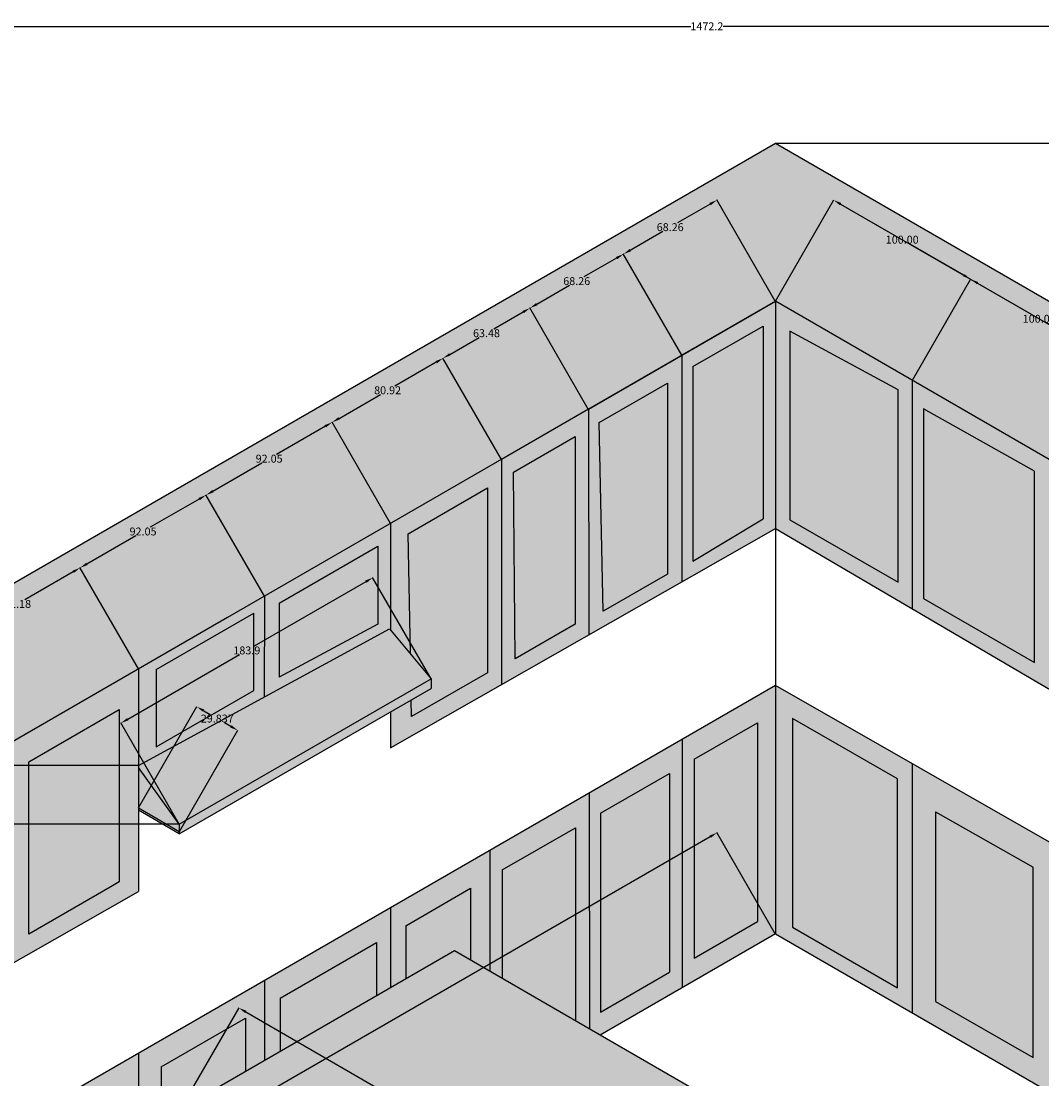
# Model space of a CAD drawing. Units: centimetres. Extents: x -744 to 1642, y 210 to 1375.
# Tile 3 of 8: x -357 to 288, y 707 to 1375. Entities that reach past the tile are written whole.
import ezdxf

# ---------------------------------------------------------------- set-up
doc = ezdxf.new("R2010")
doc.units = ezdxf.units.CM
doc.header["$MEASUREMENT"] = 0
for name, color, linetype, lineweight in [('A-ANNO-DIMS', 2, 'Continuous', 18), ('A-EQPM-PATT', 9, 'Continuous', 13), ('A-FURN', 7, 'Continuous', 25), ('A-FURN-PATT', 30, 'Continuous', 13), ('A-WALL-PATT', 61, 'Continuous', 13)]:
    doc.layers.add(name, color=color, linetype=linetype, lineweight=lineweight)
doc.styles.get("Standard").update_dxf_attribs({"font": 'arial.ttf'})
doc.dimstyles.get("Standard").update_dxf_attribs({"dimtxt": 5, "dimasz": 5, "dimexe": 0.18, "dimexo": 0.0625, "dimgap": 0.09, "dimtad": 0, "dimtih": 1, "dimtoh": 1, "dimdec": 0, "dimzin": 0, "dimdsep": 46, "dimtxsty": 'Standard', "dimcen": 0.09, "dimadec": 0, "dimazin": 0, "dimtfac": 1, "dimtdec": 0, "dimtofl": 0, "dimtmove": 0, "dimatfit": 3, "dimfxl": 1, "dimtolj": 1, "dimtzin": 0, "dimarcsym": 0})

# ---------------------------------------------------------------- blocks, each defined once
blk = doc.blocks.new('*D7')
at = {"layer": 'A-ANNO-DIMS', "color": 0, "lineweight": -2, "transparency": 16777216}
for p, q in [((-659.99, 848.29), (-659.99, 1372.26)), ((-654.99, 1372.08), (65.92, 1372.08)), ((807.25, 1372.08), (86.34, 1372.08)), ((812.25, 898.29), (812.25, 1372.26))]:
    blk.add_line(p, q, dxfattribs=at)
at = {"layer": 'A-ANNO-DIMS', "color": 0, "transparency": 16777216}
for points in [[(-654.99, 1372.91), (-654.99, 1371.25), (-659.99, 1372.08)], [(807.25, 1372.91), (807.25, 1371.25), (812.25, 1372.08)]]:
    blk.add_solid(points, dxfattribs=at)
at = {"layer": 'Defpoints', "color": 0, "transparency": 16777216}
for p in [(812.25, 1372.08), (812.25, 898.23), (-659.99, 848.23)]:
    blk.add_point(p, dxfattribs=at)
at = {"layer": 'A-ANNO-DIMS', "color": 0, "transparency": 16777216, "insert": (76.13, 1372.08), "char_height": 5, "attachment_point": 5}
blk.add_mtext('\\A1;1472.2', dxfattribs=at)
blk = doc.blocks.new('*D10')
at = {"layer": 'A-ANNO-DIMS', "color": 0, "lineweight": -2, "transparency": 16777216}
for p, q in [((119.5, 1298.23), (886.28, 1298.23)), ((886.1, 1293.23), (886.1, 795.5)), ((886.1, 292.48), (886.1, 790.21)), ((89.78, 287.48), (886.28, 287.48))]:
    blk.add_line(p, q, dxfattribs=at)
at = {"layer": 'A-ANNO-DIMS', "color": 0, "transparency": 16777216}
for points in [[(885.27, 1293.23), (886.94, 1293.23), (886.1, 1298.23)], [(885.27, 292.48), (886.94, 292.48), (886.1, 287.48)]]:
    blk.add_solid(points, dxfattribs=at)
at = {"layer": 'Defpoints', "color": 0, "transparency": 16777216}
for p in [(119.43, 1298.23), (886.1, 1298.23), (89.72, 287.48)]:
    blk.add_point(p, dxfattribs=at)
at = {"layer": 'A-ANNO-DIMS', "color": 0, "transparency": 16777216, "insert": (886.1, 792.86), "char_height": 5, "attachment_point": 5}
blk.add_mtext('\\A1;1010.7', dxfattribs=at)
blk = doc.blocks.new('*D16')
at = {"layer": 'A-ANNO-DIMS', "color": 0, "lineweight": -2, "transparency": 16777216}
for p, q in [((78.18, 859.69), (-259.32, 664.83)), ((119.4, 798.28), (82.42, 862.34)), ((-605.98, 464.69), (-268.48, 659.54)), ((-573.42, 398.28), (-610.4, 462.34))]:
    blk.add_line(p, q, dxfattribs=at)
at = {"layer": 'A-ANNO-DIMS', "color": 0, "transparency": 16777216}
for points in [[(77.76, 860.41), (78.6, 858.97), (82.51, 862.19)], [(-606.4, 465.41), (-605.57, 463.97), (-610.31, 462.19)]]:
    blk.add_solid(points, dxfattribs=at)
at = {"layer": 'Defpoints', "color": 0, "transparency": 16777216}
for p in [(82.51, 862.19), (119.43, 798.23), (-573.39, 398.23)]:
    blk.add_point(p, dxfattribs=at)
at = {"layer": 'A-ANNO-DIMS', "color": 0, "transparency": 16777216, "insert": (-263.9, 662.19), "char_height": 5, "attachment_point": 5}
blk.add_mtext('\\A1;800', dxfattribs=at)
blk = doc.blocks.new('*D17')
at = {"layer": 'A-ANNO-DIMS', "color": 0, "lineweight": -2, "transparency": 16777216}
for p, q in [((119.46, 1198.28), (156.45, 1262.34)), ((160.69, 1259.69), (454.89, 1089.83)), ((758.25, 914.69), (464.04, 1084.54)), ((725.68, 848.28), (762.67, 912.34))]:
    blk.add_line(p, q, dxfattribs=at)
at = {"layer": 'A-ANNO-DIMS', "color": 0, "transparency": 16777216}
for points in [[(161.11, 1260.41), (160.27, 1258.97), (156.36, 1262.19)], [(758.66, 915.41), (757.83, 913.97), (762.58, 912.19)]]:
    blk.add_solid(points, dxfattribs=at)
at = {"layer": 'Defpoints', "color": 0, "transparency": 16777216}
for p in [(119.43, 1198.23), (762.58, 912.19), (725.65, 848.23)]:
    blk.add_point(p, dxfattribs=at)
at = {"layer": 'A-ANNO-DIMS', "color": 0, "transparency": 16777216, "insert": (459.47, 1087.19), "char_height": 5, "attachment_point": 5}
blk.add_mtext('\\A1;700', dxfattribs=at)
blk = doc.blocks.new('*D21')
at = {"layer": 'A-ANNO-DIMS', "color": 0, "lineweight": -2, "transparency": 16777216}
for p, q in [((-98.21, 959.56), (-135.19, 1023.61)), ((-139.43, 1020.96), (-210.16, 980.13)), ((-290.04, 934.01), (-219.32, 974.84)), ((-257.47, 867.61), (-294.46, 931.66))]:
    blk.add_line(p, q, dxfattribs=at)
at = {"layer": 'A-ANNO-DIMS', "color": 0, "transparency": 16777216}
for points in [[(-139.85, 1021.68), (-139.02, 1020.24), (-135.1, 1023.46)], [(-290.45, 934.73), (-289.62, 933.29), (-294.37, 931.51)]]:
    blk.add_solid(points, dxfattribs=at)
at = {"layer": 'Defpoints', "color": 0, "transparency": 16777216}
for p in [(-135.1, 1023.46), (-98.18, 959.5), (-257.44, 867.55)]:
    blk.add_point(p, dxfattribs=at)
at = {"layer": 'A-ANNO-DIMS', "color": 0, "transparency": 16777216, "insert": (-214.74, 977.48), "char_height": 5, "attachment_point": 5}
blk.add_mtext('\\A1;183.9', dxfattribs=at)
blk = doc.blocks.new('*D22')
at = {"layer": 'A-ANNO-DIMS', "color": 0, "lineweight": -2, "transparency": 16777216}
for p, q in [((-283.34, 904.75), (-734.02, 904.75)), ((-733.84, 899.75), (-733.84, 888.8)), ((-733.84, 872.55), (-733.84, 883.51)), ((-257.51, 867.55), (-734.02, 867.55))]:
    blk.add_line(p, q, dxfattribs=at)
at = {"layer": 'A-ANNO-DIMS', "color": 0, "transparency": 16777216}
for points in [[(-734.67, 899.75), (-733.01, 899.75), (-733.84, 904.75)], [(-734.67, 872.55), (-733.01, 872.55), (-733.84, 867.55)]]:
    blk.add_solid(points, dxfattribs=at)
at = {"layer": 'Defpoints', "color": 0, "transparency": 16777216}
for p in [(-283.28, 904.75), (-733.84, 867.55), (-257.44, 867.55)]:
    blk.add_point(p, dxfattribs=at)
at = {"layer": 'A-ANNO-DIMS', "color": 0, "transparency": 16777216, "insert": (-733.84, 886.15), "char_height": 5, "attachment_point": 5}
blk.add_mtext('\\A1;37.2', dxfattribs=at)
blk = doc.blocks.new('*D23')
at = {"layer": 'A-ANNO-DIMS', "color": 0, "lineweight": -2, "transparency": 16777216}
for p, q in [((-256.66, 687.54), (-219.67, 751.59)), ((-215.43, 748.94), (-51.14, 654.08)), ((122.32, 553.94), (-41.98, 648.79)), ((89.75, 487.54), (126.74, 551.59))]:
    blk.add_line(p, q, dxfattribs=at)
at = {"layer": 'A-ANNO-DIMS', "color": 0, "transparency": 16777216}
for points in [[(-215.02, 749.66), (-215.85, 748.22), (-219.76, 751.44)], [(122.73, 554.66), (121.9, 553.22), (126.65, 551.44)]]:
    blk.add_solid(points, dxfattribs=at)
at = {"layer": 'Defpoints', "color": 0, "transparency": 16777216}
for p in [(-256.69, 687.48), (126.65, 551.44), (89.72, 487.48)]:
    blk.add_point(p, dxfattribs=at)
at = {"layer": 'A-ANNO-DIMS', "color": 0, "transparency": 16777216, "insert": (-46.56, 651.44), "char_height": 5, "attachment_point": 5}
blk.add_mtext('\\A1;400', dxfattribs=at)
blk = doc.blocks.new('*D45')
at = {"layer": 'A-ANNO-DIMS', "color": 0, "lineweight": -2, "transparency": 16777216}
for p, q in [((-324.54, 1027.18), (-355.11, 1009.53)), ((-283.31, 965.78), (-320.3, 1029.83)), ((-394.84, 986.59), (-364.27, 1004.24)), ((-362.28, 920.19), (-399.26, 984.25))]:
    blk.add_line(p, q, dxfattribs=at)
at = {"layer": 'A-ANNO-DIMS', "color": 0, "transparency": 16777216}
for points in [[(-324.95, 1027.9), (-324.12, 1026.46), (-320.21, 1029.68)], [(-395.26, 987.31), (-394.42, 985.87), (-399.17, 984.09)]]:
    blk.add_solid(points, dxfattribs=at)
at = {"layer": 'Defpoints', "color": 0, "transparency": 16777216}
for p in [(-320.21, 1029.68), (-283.28, 965.72), (-362.24, 920.13)]:
    blk.add_point(p, dxfattribs=at)
at = {"layer": 'A-ANNO-DIMS', "color": 0, "transparency": 16777216, "insert": (-359.69, 1006.88), "char_height": 5, "attachment_point": 5}
blk.add_mtext('\\A1;91.18', dxfattribs=at)
blk = doc.blocks.new('*D46')
at = {"layer": 'A-ANNO-DIMS', "color": 0, "lineweight": -2, "transparency": 16777216}
for p, q in [((-244.82, 1073.2), (-275.77, 1055.33)), ((-203.6, 1011.8), (-240.58, 1075.86)), ((-315.88, 1032.18), (-284.93, 1050.05)), ((-283.31, 965.78), (-320.3, 1029.83))]:
    blk.add_line(p, q, dxfattribs=at)
at = {"layer": 'A-ANNO-DIMS', "color": 0, "transparency": 16777216}
for points in [[(-245.24, 1073.92), (-244.4, 1072.48), (-240.49, 1075.7)], [(-316.29, 1032.9), (-315.46, 1031.46), (-320.21, 1029.68)]]:
    blk.add_solid(points, dxfattribs=at)
at = {"layer": 'Defpoints', "color": 0, "transparency": 16777216}
for p in [(-240.49, 1075.7), (-203.57, 1011.75), (-283.28, 965.72)]:
    blk.add_point(p, dxfattribs=at)
at = {"layer": 'A-ANNO-DIMS', "color": 0, "transparency": 16777216, "insert": (-280.35, 1052.69), "char_height": 5, "attachment_point": 5}
blk.add_mtext('\\A1;92.05', dxfattribs=at)
blk = doc.blocks.new('*D47')
at = {"layer": 'A-ANNO-DIMS', "color": 0, "lineweight": -2, "transparency": 16777216}
for p, q in [((-165.1, 1119.23), (-196.05, 1101.36)), ((-123.88, 1057.83), (-160.86, 1121.88)), ((-236.16, 1078.2), (-205.21, 1096.07)), ((-203.6, 1011.8), (-240.58, 1075.86))]:
    blk.add_line(p, q, dxfattribs=at)
at = {"layer": 'A-ANNO-DIMS', "color": 0, "transparency": 16777216}
for points in [[(-165.52, 1119.95), (-164.69, 1118.51), (-160.77, 1121.73)], [(-236.58, 1078.92), (-235.74, 1077.48), (-240.49, 1075.7)]]:
    blk.add_solid(points, dxfattribs=at)
at = {"layer": 'Defpoints', "color": 0, "transparency": 16777216}
for p in [(-160.77, 1121.73), (-123.85, 1057.77), (-203.57, 1011.75)]:
    blk.add_point(p, dxfattribs=at)
at = {"layer": 'A-ANNO-DIMS', "color": 0, "transparency": 16777216, "insert": (-200.63, 1098.72), "char_height": 5, "attachment_point": 5}
blk.add_mtext('\\A1;92.05', dxfattribs=at)
blk = doc.blocks.new('*D48')
at = {"layer": 'A-ANNO-DIMS', "color": 0, "lineweight": -2, "transparency": 16777216}
for p, q in [((-95.03, 1159.69), (-121.16, 1144.6)), ((-53.8, 1098.28), (-90.79, 1162.34)), ((-156.44, 1124.23), (-130.31, 1139.31)), ((-123.88, 1057.83), (-160.86, 1121.88))]:
    blk.add_line(p, q, dxfattribs=at)
at = {"layer": 'A-ANNO-DIMS', "color": 0, "transparency": 16777216}
for points in [[(-95.44, 1160.41), (-94.61, 1158.97), (-90.7, 1162.19)], [(-156.86, 1124.95), (-156.03, 1123.51), (-160.77, 1121.73)]]:
    blk.add_solid(points, dxfattribs=at)
at = {"layer": 'Defpoints', "color": 0, "transparency": 16777216}
for p in [(-90.7, 1162.19), (-53.77, 1098.23), (-123.85, 1057.77)]:
    blk.add_point(p, dxfattribs=at)
at = {"layer": 'A-ANNO-DIMS', "color": 0, "transparency": 16777216, "insert": (-125.74, 1141.96), "char_height": 5, "attachment_point": 5}
blk.add_mtext('\\A1;80.92', dxfattribs=at)
blk = doc.blocks.new('*D49')
at = {"layer": 'A-ANNO-DIMS', "color": 0, "lineweight": -2, "transparency": 16777216}
for p, q in [((-40.05, 1191.43), (-58.63, 1180.7)), ((1.17, 1130.02), (-35.81, 1194.08)), ((-86.37, 1164.69), (-67.79, 1175.41)), ((-53.8, 1098.28), (-90.79, 1162.34))]:
    blk.add_line(p, q, dxfattribs=at)
at = {"layer": 'A-ANNO-DIMS', "color": 0, "transparency": 16777216}
for points in [[(-40.47, 1192.15), (-39.64, 1190.7), (-35.72, 1193.93)], [(-86.78, 1165.41), (-85.95, 1163.97), (-90.7, 1162.19)]]:
    blk.add_solid(points, dxfattribs=at)
at = {"layer": 'Defpoints', "color": 0, "transparency": 16777216}
for p in [(-35.72, 1193.93), (1.2, 1129.97), (-53.77, 1098.23)]:
    blk.add_point(p, dxfattribs=at)
at = {"layer": 'A-ANNO-DIMS', "color": 0, "transparency": 16777216, "insert": (-63.21, 1178.06), "char_height": 5, "attachment_point": 5}
blk.add_mtext('\\A1;63.48', dxfattribs=at)
blk = doc.blocks.new('*D50')
at = {"layer": 'A-ANNO-DIMS', "color": 0, "lineweight": -2, "transparency": 16777216}
for p, q in [((19.06, 1225.56), (-1.59, 1213.63)), ((60.29, 1164.15), (23.3, 1228.21)), ((-31.39, 1196.43), (-10.74, 1208.35)), ((1.17, 1130.02), (-35.81, 1194.08))]:
    blk.add_line(p, q, dxfattribs=at)
at = {"layer": 'A-ANNO-DIMS', "color": 0, "transparency": 16777216}
for points in [[(18.65, 1226.28), (19.48, 1224.83), (23.39, 1228.06)], [(-31.81, 1197.15), (-30.98, 1195.7), (-35.72, 1193.93)]]:
    blk.add_solid(points, dxfattribs=at)
at = {"layer": 'Defpoints', "color": 0, "transparency": 16777216}
for p in [(23.39, 1228.06), (60.32, 1164.1), (1.2, 1129.97)]:
    blk.add_point(p, dxfattribs=at)
at = {"layer": 'A-ANNO-DIMS', "color": 0, "transparency": 16777216, "insert": (-6.17, 1210.99), "char_height": 5, "attachment_point": 5}
blk.add_mtext('\\A1;68.26', dxfattribs=at)
blk = doc.blocks.new('*D51')
at = {"layer": 'A-ANNO-DIMS', "color": 0, "lineweight": -2, "transparency": 16777216}
for p, q in [((78.18, 1259.69), (57.53, 1247.76)), ((119.4, 1198.28), (82.42, 1262.34)), ((27.72, 1230.56), (48.37, 1242.48)), ((60.29, 1164.15), (23.3, 1228.21))]:
    blk.add_line(p, q, dxfattribs=at)
at = {"layer": 'A-ANNO-DIMS', "color": 0, "transparency": 16777216}
for points in [[(77.76, 1260.41), (78.6, 1258.97), (82.51, 1262.19)], [(27.31, 1231.28), (28.14, 1229.83), (23.39, 1228.06)]]:
    blk.add_solid(points, dxfattribs=at)
at = {"layer": 'Defpoints', "color": 0, "transparency": 16777216}
for p in [(82.51, 1262.19), (119.43, 1198.23), (60.32, 1164.1)]:
    blk.add_point(p, dxfattribs=at)
at = {"layer": 'A-ANNO-DIMS', "color": 0, "transparency": 16777216, "insert": (52.95, 1245.12), "char_height": 5, "attachment_point": 5}
blk.add_mtext('\\A1;68.26', dxfattribs=at)
blk = doc.blocks.new('*D52')
at = {"layer": 'A-ANNO-DIMS', "color": 0, "lineweight": -2, "transparency": 16777216}
for p, q in [((119.46, 1198.28), (156.45, 1262.34)), ((160.69, 1259.69), (195.08, 1239.83)), ((238.63, 1214.69), (204.24, 1234.54)), ((206.07, 1148.28), (243.05, 1212.34))]:
    blk.add_line(p, q, dxfattribs=at)
at = {"layer": 'A-ANNO-DIMS', "color": 0, "transparency": 16777216}
for points in [[(161.11, 1260.41), (160.27, 1258.97), (156.36, 1262.19)], [(239.05, 1215.41), (238.21, 1213.97), (242.96, 1212.19)]]:
    blk.add_solid(points, dxfattribs=at)
at = {"layer": 'Defpoints', "color": 0, "transparency": 16777216}
for p in [(242.96, 1212.19), (119.43, 1198.23), (206.04, 1148.23)]:
    blk.add_point(p, dxfattribs=at)
at = {"layer": 'A-ANNO-DIMS', "color": 0, "transparency": 16777216, "insert": (199.66, 1237.19), "char_height": 5, "attachment_point": 5}
blk.add_mtext('\\A1;100.00', dxfattribs=at)
blk = doc.blocks.new('*D53')
at = {"layer": 'A-ANNO-DIMS', "color": 0, "lineweight": -2, "transparency": 16777216}
for p, q in [((206.07, 1148.28), (243.05, 1212.34)), ((247.29, 1209.69), (281.68, 1189.83)), ((325.23, 1164.69), (290.84, 1184.54)), ((292.67, 1098.28), (329.65, 1162.34))]:
    blk.add_line(p, q, dxfattribs=at)
at = {"layer": 'A-ANNO-DIMS', "color": 0, "transparency": 16777216}
for points in [[(247.71, 1210.41), (246.87, 1208.97), (242.96, 1212.19)], [(325.65, 1165.41), (324.82, 1163.97), (329.56, 1162.19)]]:
    blk.add_solid(points, dxfattribs=at)
at = {"layer": 'Defpoints', "color": 0, "transparency": 16777216}
for p in [(329.56, 1162.19), (206.04, 1148.23), (292.64, 1098.23)]:
    blk.add_point(p, dxfattribs=at)
at = {"layer": 'A-ANNO-DIMS', "color": 0, "transparency": 16777216, "insert": (286.26, 1187.19), "char_height": 5, "attachment_point": 5}
blk.add_mtext('\\A1;100.00', dxfattribs=at)
blk = doc.blocks.new('*D58')
at = {"layer": 'A-ANNO-DIMS', "color": 0, "lineweight": -2, "transparency": 16777216}
for p, q in [((-283.25, 877.97), (-246.27, 942.03)), ((-242.03, 939.37), (-238.02, 937.06)), ((-224.85, 929.45), (-228.86, 931.77)), ((-257.41, 863.05), (-220.43, 927.11))]:
    blk.add_line(p, q, dxfattribs=at)
at = {"layer": 'A-ANNO-DIMS', "color": 0, "transparency": 16777216}
for points in [[(-241.61, 940.09), (-242.44, 938.65), (-246.36, 941.87)], [(-224.43, 930.18), (-225.26, 928.73), (-220.52, 926.95)]]:
    blk.add_solid(points, dxfattribs=at)
at = {"layer": 'Defpoints', "color": 0, "transparency": 16777216}
for p in [(-220.52, 926.95), (-283.28, 877.92), (-257.44, 863)]:
    blk.add_point(p, dxfattribs=at)
at = {"layer": 'A-ANNO-DIMS', "color": 0, "transparency": 16777216, "insert": (-233.44, 934.41), "char_height": 5, "attachment_point": 5}
blk.add_mtext('\\A1;29.837', dxfattribs=at)

msp = doc.modelspace()

# ---------------------------------------------------------------- hatches: boundary and pattern name
at = {"layer": 'A-EQPM-PATT'}
h = msp.add_hatch(color=256, dxfattribs=at)
h.dxf.hatch_style = 1
h.paths.add_polyline_path([(-98.1787, 959.5025), (-124.4818, 991.1041), (-283.2822, 904.7538), (-283.2822, 903.5283), (-257.4428, 867.552)])
h.paths.add_polyline_path([(-283.2822, 903.5283), (-283.2822, 877.9161), (-257.4428, 862.9977), (-257.4428, 867.552)])
h.paths.add_polyline_path([(-98.1787, 953.5165), (-98.1787, 959.5025), (-257.4428, 867.552), (-257.4428, 862.9977), (-257.4428, 861.5653)])
h.paths.add_polyline_path([(595.7475, 816.0455), (465.8437, 891.6699), (465.8437, 699.3662), (595.7475, 624.3662)])
h.paths.add_polyline_path([(579.2833, 788.737), (583.6533, 785.4908), (583.6533, 654.1832), (579.2833, 656.7062)], flags=16)
h.paths.add_polyline_path([(725.6513, 740.4211), (595.7475, 816.0455), (595.7475, 624.3662), (725.6513, 549.3662)])
h.paths.add_polyline_path([(610.2064, 643.0466), (605.8363, 645.5696), (605.8363, 777.6004), (610.2064, 774.3542)], flags=16)
h.paths.add_polyline_path([(595.7475, 624.3662), (465.8437, 699.3662), (465.8437, 598.2308), (725.6513, 448.2308), (725.6513, 549.3662)])
h = msp.add_hatch(color=256, dxfattribs=at)
h.dxf.hatch_style = 1
h.paths.add_polyline_path([(3.1189, 737.4813), (-83.4836, 787.4813), (-256.6887, 687.4813), (89.7215, 487.4813), (262.9266, 587.4813)])
h.paths.add_polyline_path([(-197.7282, 644.2029), (-248.6887, 673.6249), (-248.6887, 482.8625), (-196.7272, 512.8625)])
h.paths.add_polyline_path([(262.9266, 587.4813), (89.7215, 487.4813), (89.7215, 287.4813), (262.9266, 387.4813)])
at = {"layer": 'A-FURN-PATT'}
h = msp.add_hatch(color=256, dxfattribs=at)
h.dxf.hatch_style = 1
h.paths.add_polyline_path([(709.906, 763.421), (709.906, 833.5619), (614.425, 888.6879), (614.425, 818.5469)])
h.paths.add_polyline_path([(482.0889, 965.0922), (482.0889, 894.9512), (580.3491, 838.2207), (580.3491, 908.3616)])
h.paths.add_polyline_path([(455.661, 989.3482), (391.7403, 1026.2528), (391.7403, 905.908), (455.661, 869.0034)])
h.paths.add_polyline_path([(367.6025, 1038.9798), (305.4698, 1074.8522), (305.4698, 959.5913), (367.6025, 923.719)])
h.paths.add_polyline_path([(283.2252, 1090.8212), (213.1748, 1130.1519), (213.1748, 1010.3029), (283.2252, 969.8593)])
h.paths.add_polyline_path([(197.085, 1142.1995), (128.5906, 1179.2565), (128.5906, 1060.1567), (197.085, 1020.6114)])
h.paths.add_polyline_path([(111.6616, 1060.697), (111.6616, 1182.612), (67.1993, 1156.9417), (67.1993, 1033.9561)])
h.paths.add_polyline_path([(51.1364, 1025.5999), (51.1364, 1146.3882), (8.133, 1121.5602), (10.63, 1002.2135)])
h.paths.add_polyline_path([(-7.1228, 994.0363), (-7.1228, 1112.7639), (-46.1416, 1090.2363), (-45.0502, 972.1389)])
h.paths.add_polyline_path([(-62.5525, 1080.1953), (-112.7586, 1051.2088), (-111.3243, 975.2962), (-98.1787, 959.5025), (-98.1787, 953.5165), (-110.7754, 946.2438), (-110.5757, 935.6761), (-62.5525, 963.4023)])
h.paths.add_polyline_path([(-131.9167, 1043.3731), (-194.3022, 1007.3548), (-194.3022, 960.6093), (-131.9167, 994.0283)])
h.paths.add_polyline_path([(-210.3768, 1001.0803), (-272.1227, 965.4313), (-272.1227, 916.524), (-210.3442, 952.1919)])
h.paths.add_polyline_path([(-295.3923, 940.164), (-352.6194, 907.1238), (-352.6194, 798.1578), (-299.691, 828.716), (-295.3923, 831.1979)])
h.paths.add_polyline_path([(-373.8641, 892.8311), (-430.554, 860.1012), (-428.9419, 756.8396), (-373.8641, 788.6388)])
h.paths.add_polyline_path([(-449.1461, 850.3626), (-500.1893, 820.8928), (-498.1887, 714.0073), (-449.1461, 742.322)])
h.paths.add_polyline_path([(-517.3336, 813.4139), (-562.861, 787.1286), (-563.3952, 675.4493), (-517.3336, 702.043)])
h.paths.add_polyline_path([(-518.4603, 570.0519), (-562.9383, 544.3726), (-563.4408, 418.3375), (-518.4603, 444.307)])
h.paths.add_polyline_path([(-371.5223, 654.8866), (-429.2034, 621.5845), (-429.2034, 495.8395), (-371.5223, 529.1417)])
h.paths.add_polyline_path([(-448.7547, 610.2965), (-500.7971, 580.2498), (-501.5895, 454.0473), (-449.5067, 484.1173)])
h.paths.add_polyline_path([(-351.4436, 666.4791), (-351.4436, 540.7341), (-295.2328, 573.1874), (-295.2328, 698.9324)])
h.paths.add_polyline_path([(-256.6887, 595.4409), (-256.6887, 687.4813), (-215.6652, 711.1662), (-215.6652, 744.8707), (-268.9239, 714.1219), (-268.9239, 588.3769)])
h.paths.add_polyline_path([(-193.7313, 723.8298), (-132.6965, 759.0682), (-132.6965, 792.7727), (-193.7313, 757.5343)])
h.paths.add_polyline_path([(-114.2, 769.7472), (-83.4836, 787.4813), (-73.2438, 781.5694), (-73.2438, 827.0978), (-114.2, 803.4517)])
h.paths.add_polyline_path([(-53.2271, 770.0128), (-7.0224, 743.3364), (-7.0224, 865.3308), (-53.2271, 838.6544)])
h.paths.add_polyline_path([(8.89, 748.7728), (52.5303, 773.9686), (52.5303, 899.7135), (8.89, 874.5177)])
h.paths.add_polyline_path([(68.067, 782.9387), (108.041, 806.0177), (108.041, 931.7626), (68.067, 908.6836)])
h.paths.add_polyline_path([(130.3442, 802.4419), (196.727, 764.1157), (196.727, 896.2228), (130.3442, 934.5489), (130.3442, 927.6391)])
h.paths.add_polyline_path([(220.7637, 875.3463), (220.7637, 755.5756), (282.3763, 720.0036), (282.3763, 835.7573), (282.3763, 840.4873)])
h.paths.add_polyline_path([(307.3754, 826.3434), (307.3754, 705.693), (368.1078, 670.6291), (368.1078, 790.9456)])
h.paths.add_polyline_path([(389.5829, 779.9795), (389.5829, 656.983), (453.252, 620.2237), (453.252, 747.8082)])
at = {"layer": 'A-WALL-PATT'}
h = msp.add_hatch(color=256, dxfattribs=at)
h.dxf.hatch_style = 1
h.paths.add_polyline_path([(-226.9766, 998.2308), (119.4335, 1198.2308), (292.6386, 1098.2308), (465.8437, 998.2308), (552.4462, 948.2308), (725.6513, 848.2308), (812.2538, 898.2308), (119.4335, 1298.2308), (-659.9893, 848.2308), (-573.3868, 798.2308)])
h.paths.add_polyline_path([(-573.3868, 798.2308), (-659.9893, 848.2308), (-659.9893, 448.2308), (-573.3868, 398.2308)])
h.paths.add_polyline_path([(-507.2972, 836.3877), (-573.3868, 798.2308), (-573.3868, 659.7809), (-507.2972, 697.4412)])
h.paths.add_polyline_path([(-562.861, 787.1286), (-517.3336, 813.4139), (-517.3336, 702.043), (-563.3952, 675.4493)], flags=16)
h.paths.add_polyline_path([(-441.2075, 735.1015), (-441.2075, 874.5446), (-507.2972, 836.3877), (-507.2972, 697.4412)])
h.paths.add_polyline_path([(-500.1893, 820.8928), (-449.1461, 850.3626), (-449.1461, 742.322), (-498.1887, 714.0073)], flags=16)
h.paths.add_polyline_path([(-362.2449, 780.0973), (-362.2449, 920.1337), (-441.2075, 874.5446), (-441.2075, 735.1015)])
h.paths.add_polyline_path([(-430.554, 860.1012), (-373.8641, 892.8311), (-373.8641, 788.6388), (-428.9419, 756.8396)], flags=16)
h.paths.add_polyline_path([(-283.2822, 825.0931), (-283.2822, 965.7228), (-362.2449, 920.1337), (-362.2449, 780.0973)])
h.paths.add_polyline_path([(-352.6194, 798.1578), (-352.6194, 907.1238), (-295.3923, 940.164), (-295.3923, 831.1979), (-299.691, 828.716)], flags=16)
h.paths.add_polyline_path([(-203.882, 947.929), (-203.5655, 1011.7473), (-226.9766, 998.2308), (-283.2822, 965.7228), (-283.2822, 904.7538)], flags=17)
h.paths.add_polyline_path([(-272.1227, 965.4313), (-210.3768, 1001.0803), (-210.3442, 952.1919), (-272.1227, 916.524)], flags=16)
h.paths.add_polyline_path([(-123.8488, 991.4483), (-123.8488, 1057.7717), (-203.5655, 1011.7473), (-203.882, 947.929)], flags=17)
h.paths.add_polyline_path([(-194.3022, 1007.3548), (-131.9167, 1043.3731), (-131.9167, 994.0283), (-194.3022, 960.6093)], flags=16)
h.paths.add_polyline_path([(-112.7586, 1051.2088), (-62.5525, 1080.1953), (-62.5525, 963.4023), (-110.5757, 935.6761), (-110.7754, 946.2438), (-123.8488, 938.6959), (-123.8488, 915.9442), (-53.7716, 955.8768), (-53.7716, 1098.2308), (-123.8488, 1057.7717), (-123.8488, 991.4483), (-123.8488, 990.3436), (-111.3243, 975.2962)], flags=17)
h.paths.add_polyline_path([(1.2011, 1129.9693), (-53.7716, 1098.2308), (-53.7716, 955.8768), (1.4435, 987.3403)], flags=17)
h.paths.add_polyline_path([(-46.1416, 1090.2363), (-7.1228, 1112.7639), (-7.1228, 994.0363), (-45.0502, 972.1389)], flags=16)
h.paths.add_polyline_path([(60.3173, 1164.1001), (1.2011, 1129.9693), (1.4435, 987.3403), (60.3173, 1020.8888)], flags=17)
h.paths.add_polyline_path([(8.133, 1121.5602), (51.1364, 1146.3882), (51.1364, 1025.5999), (10.63, 1002.2135)], flags=16)
h.paths.add_polyline_path([(119.4335, 1054.5754), (119.4335, 1198.2308), (60.3173, 1164.1001), (60.3173, 1020.8888)], flags=17)
h.paths.add_polyline_path([(67.1993, 1156.9417), (111.6616, 1182.612), (111.6616, 1060.697), (67.1993, 1033.9561)], flags=16)
h.paths.add_polyline_path([(206.0361, 1148.2308), (119.4335, 1198.2308), (119.4335, 1054.5754), (206.0361, 1003.7675)], flags=17)
h.paths.add_polyline_path([(128.5906, 1179.2565), (197.085, 1142.1995), (197.085, 1020.6114), (128.5906, 1060.1567)], flags=16)
h.paths.add_polyline_path([(206.0361, 1148.2308), (206.0361, 1003.7675), (292.6386, 952.9596), (292.6386, 1098.2308)], flags=17)
h.paths.add_polyline_path([(213.1748, 1130.1519), (283.2252, 1090.8212), (283.2252, 969.8593), (213.1748, 1010.3029)], flags=16)
h.paths.add_polyline_path([(292.6386, 1098.2308), (292.6386, 952.9596), (378.4066, 902.6412), (379.2411, 1048.2308)], flags=17)
h.paths.add_polyline_path([(305.4698, 1074.8522), (367.6025, 1038.9798), (367.6025, 923.719), (305.4698, 959.5913)], flags=16)
h.paths.add_polyline_path([(379.2411, 1048.2308), (378.4066, 902.6412), (465.8437, 851.3437), (465.8437, 998.2308)], flags=17)
h.paths.add_polyline_path([(391.7403, 1026.2528), (455.661, 989.3482), (455.661, 869.0034), (391.7403, 905.908)], flags=16)
h.paths.add_polyline_path([(552.4462, 948.2308), (465.8437, 998.2308), (465.8437, 891.6699), (595.7475, 816.0455), (595.7475, 923.2308)], flags=17)
h.paths.add_polyline_path([(482.0889, 965.0922), (580.3491, 908.3616), (580.3491, 838.2207), (482.0889, 894.9512)], flags=16)
h.paths.add_polyline_path([(595.7475, 923.2308), (595.7475, 816.0455), (725.6513, 740.4211), (725.6513, 848.2308)])
h.paths.add_polyline_path([(614.425, 888.6879), (709.906, 833.5619), (709.906, 763.421), (614.425, 818.5469)], flags=16)
h.paths.add_polyline_path([(812.2538, 898.2308), (725.6513, 848.2308), (725.6513, 740.4211), (725.6513, 448.2308), (812.2538, 498.2308)])
h.paths.add_polyline_path([(465.8437, 757.085), (377.8609, 807.4399), (376.9558, 649.5503), (465.8437, 598.2308)])
h.paths.add_polyline_path([(389.5829, 779.9795), (453.252, 747.8082), (453.252, 620.2237), (389.5829, 656.983)], flags=16)
h.paths.add_polyline_path([(377.8609, 807.4399), (292.6386, 856.215), (292.6386, 698.2308), (376.9558, 649.5503)])
h.paths.add_polyline_path([(368.1078, 670.6291), (307.3754, 705.693), (307.3754, 826.3434), (368.1078, 790.9456)], flags=16)
h.paths.add_polyline_path([(292.6386, 856.215), (206.0361, 905.7799), (206.0361, 748.2308), (292.6386, 698.2308)])
h.paths.add_polyline_path([(282.3763, 720.0036), (220.7637, 755.5756), (220.7637, 875.3463), (282.3763, 840.4873), (282.3763, 835.7573)], flags=16)
h.paths.add_polyline_path([(206.0361, 905.7799), (119.4335, 955.3449), (119.4335, 798.2308), (206.0361, 748.2308)])
h.paths.add_polyline_path([(196.727, 764.1157), (130.3442, 802.4419), (130.3442, 927.6391), (130.3442, 934.5489), (196.727, 896.2228)], flags=16)
h.paths.add_polyline_path([(119.4335, 955.3449), (60.5235, 921.3332), (60.5235, 764.2191), (119.4335, 798.2308)])
h.paths.add_polyline_path([(108.041, 806.0177), (68.067, 782.9387), (68.067, 908.6836), (108.041, 931.7626)], flags=16)
h.paths.add_polyline_path([(60.5235, 764.2191), (60.5235, 921.3332), (1.6135, 887.3215), (1.867, 738.2042), (3.1189, 737.4813), (8.6656, 734.279)])
h.paths.add_polyline_path([(8.89, 748.7728), (8.89, 874.5177), (52.5303, 899.7135), (52.5303, 773.9686)], flags=16)
h.paths.add_polyline_path([(1.6135, 887.3215), (-61.1176, 851.1036), (-61.1176, 774.5683), (-53.2271, 770.0128), (-53.2271, 838.6544), (-7.0224, 865.3308), (-7.0224, 743.3364), (1.867, 738.2042)])
h.paths.add_polyline_path([(-61.1176, 851.1036), (-123.8488, 814.8858), (-123.8488, 764.1765), (-114.2, 769.7472), (-114.2, 803.4517), (-73.2438, 827.0978), (-73.2438, 781.5694), (-61.1176, 774.5683)])
h.paths.add_polyline_path([(-132.6965, 792.7727), (-132.6965, 759.0682), (-123.8488, 764.1765), (-123.8488, 814.8858), (-203.5655, 768.8613), (-203.5655, 718.152), (-193.7313, 723.8298), (-193.7313, 757.5343)])
h.paths.add_polyline_path([(-203.5655, 768.8613), (-283.2822, 722.8369), (-283.2822, 565.7228), (-256.6887, 581.0766), (-256.6887, 595.4409), (-268.9239, 588.3769), (-268.9239, 714.1219), (-215.6652, 744.8707), (-215.6652, 711.1662), (-203.5655, 718.152)])
h.paths.add_polyline_path([(-283.2822, 722.8369), (-362.2449, 677.2477), (-362.2449, 520.1337), (-283.2822, 565.7228)])
h.paths.add_polyline_path([(-295.2328, 573.1874), (-351.4436, 540.7341), (-351.4436, 666.4791), (-295.2328, 698.9324)], flags=16)
h.paths.add_polyline_path([(-362.2449, 677.2477), (-441.2075, 631.6586), (-441.2075, 474.5446), (-362.2449, 520.1337)])
h.paths.add_polyline_path([(-371.5223, 529.1417), (-429.2034, 495.8395), (-429.2034, 621.5845), (-371.5223, 654.8866)], flags=16)
h.paths.add_polyline_path([(-441.2075, 631.6586), (-507.2972, 593.5018), (-507.2972, 436.3877), (-441.2075, 474.5446)])
h.paths.add_polyline_path([(-448.7547, 610.2965), (-449.5067, 484.1173), (-501.5895, 454.0473), (-500.7971, 580.2498)], flags=16)
h.paths.add_polyline_path([(-507.2972, 593.5018), (-573.3868, 555.3449), (-573.3868, 398.2308), (-507.2972, 436.3877)])
h.paths.add_polyline_path([(-518.4603, 570.0519), (-518.4603, 444.307), (-563.4408, 418.3375), (-562.9383, 544.3726)], flags=16)
h.paths.add_polyline_path([(-118.6694, 598.5582), (-123.6694, 601.445), (-123.6694, 488.0238), (-118.6694, 485.1326)], flags=17)
h.paths.add_polyline_path([(-113.6694, 595.6715), (-118.6694, 598.5582), (-118.6694, 485.1326), (-113.6694, 482.2413)], flags=17)
h.paths.add_polyline_path([(-12.0425, 536.9972), (-17.0425, 539.8839), (-17.0425, 426.3672), (-12.0425, 423.4759)], flags=17)
h.paths.add_polyline_path([(-17.0425, 539.8839), (-22.0425, 542.7707), (-22.0425, 429.2584), (-17.0425, 426.3672)], flags=17)
h.paths.add_polyline_path([(-256.6887, 687.4813), (-256.6887, 487.4813), (-248.6887, 482.8625), (-248.6887, 673.6249), (81.7215, 482.8625), (81.7215, 292.1001), (89.7215, 287.4813), (89.7215, 487.4813)])
h.paths.add_polyline_path([(-196.8604, 530.3463), (-196.7272, 512.8625), (81.7215, 352.1001), (81.7215, 369.2572)], flags=17)

# ---------------------------------------------------------------- linework, layer by layer
at = {"layer": 'A-FURN'}
for p, q in [((-659.9893, 848.2308), (119.4335, 1298.2308)), ((119.4335, 1298.2308), (812.2538, 898.2308)), ((119.4335, 1198.2308), (-226.9766, 998.2308)), ((1.2011, 1129.9693), (119.4335, 1198.2308)), ((119.4335, 1198.2308), (60.3173, 1164.1001)), ((292.6386, 1098.2308), (119.4335, 1198.2308)), ((119.4335, 1198.2308), (119.4335, 798.2308)), ((67.1993, 1156.9417), (111.6616, 1182.612)), ((111.6616, 1182.612), (111.6616, 1060.697)), ((128.5906, 1179.2565), (128.5906, 1060.1567)), ((197.085, 1142.1995), (128.5906, 1179.2565)), ((60.3173, 1164.1001), (60.3173, 1020.8888)), ((67.1993, 1156.9417), (67.1993, 1033.9561)), ((8.133, 1121.5602), (51.1364, 1146.3882)), ((51.1364, 1146.3882), (51.1364, 1025.5999)), ((206.0361, 1148.2308), (206.0361, 1003.7675)), ((197.085, 1020.6114), (197.085, 1142.1995)), ((1.2011, 1129.9693), (-53.7716, 1098.2308)), ((1.2011, 1129.9693), (1.4435, 987.3403)), ((213.1748, 1130.1519), (213.1748, 1010.3029)), ((283.2252, 1090.8212), (213.1748, 1130.1519)), ((10.63, 1002.2135), (8.133, 1121.5602)), ((-46.1416, 1090.2363), (-7.1228, 1112.7639)), ((-7.1228, 1112.7639), (-7.1228, 994.0363)), ((-53.7716, 1098.2308), (-53.7716, 955.8768)), ((-45.0502, 972.1389), (-46.1416, 1090.2363)), ((283.2252, 969.8593), (283.2252, 1090.8212)), ((-112.7586, 1051.2088), (-62.5525, 1080.1953)), ((-62.5525, 1080.1953), (-62.5525, 963.4023)), ((-123.8488, 1057.7717), (-123.8488, 990.3436)), ((67.1993, 1033.9561), (111.6616, 1060.697)), ((128.5906, 1060.1567), (197.085, 1020.6114)), ((-123.8488, 915.9442), (119.4335, 1054.5754)), ((-111.3243, 975.2962), (-112.7586, 1051.2088)), ((119.4335, 1054.5754), (465.8437, 851.3437)), ((-194.3022, 1007.3548), (-131.9167, 1043.3731)), ((-131.9167, 1043.3731), (-131.9167, 994.0283)), ((51.1364, 1025.5999), (10.63, 1002.2135)), ((-203.5655, 1011.7473), (-203.882, 947.929)), ((213.1748, 1010.3029), (283.2252, 969.8593)), ((-194.3022, 1007.3548), (-194.3022, 960.6093)), ((-226.9766, 998.2308), (-573.3868, 798.2308)), ((-272.1227, 965.4313), (-210.3768, 1001.0803)), ((-210.3442, 952.1919), (-210.3768, 1001.0803)), ((-283.2822, 904.7538), (-124.4818, 991.1041)), ((-131.9167, 994.0283), (-194.3022, 960.6093)), ((-124.4818, 991.1041), (-98.1787, 959.5025)), ((-7.1228, 994.0363), (-45.0502, 972.1389)), ((-283.2822, 965.7228), (-283.2822, 825.0931)), ((-272.1227, 965.4313), (-272.1227, 916.524)), ((-62.5525, 963.4023), (-110.5757, 935.6761)), ((-257.4428, 867.552), (-98.1787, 959.5025)), ((-98.1787, 959.5025), (-98.1787, 953.5165)), ((119.4335, 955.3449), (-573.3868, 555.3449)), ((-272.1227, 916.524), (-210.3442, 952.1919)), ((-257.4428, 861.5653), (-98.1787, 953.5165)), ((465.8437, 757.085), (119.4335, 955.3449)), ((-110.5757, 935.6761), (-110.7754, 946.2438)), ((-352.6194, 907.1238), (-295.3923, 940.164)), ((-295.3923, 940.164), (-295.3923, 831.1979)), ((-123.8488, 938.6959), (-123.8488, 915.9442)), ((68.067, 908.6836), (108.041, 931.7626)), ((108.041, 931.7626), (108.041, 806.0177)), ((196.727, 896.2228), (130.3442, 934.5489)), ((130.3442, 934.5489), (130.3442, 927.6391)), ((130.3442, 927.6391), (130.3442, 802.4419)), ((-123.8488, 918.5696), (-123.8488, 915.9442)), ((60.5235, 921.3332), (60.5235, 764.2191)), ((-352.6194, 798.1578), (-352.6194, 907.1238)), ((-257.4428, 867.552), (-283.2822, 903.5283)), ((68.067, 908.6836), (68.067, 782.9387)), ((206.0361, 905.7799), (206.0361, 748.2308)), ((8.89, 874.5177), (52.5303, 899.7135)), ((52.5303, 899.7135), (52.5303, 773.9686)), ((196.727, 764.1157), (196.727, 896.2228)), ((1.6135, 887.3215), (1.867, 738.2042)), ((-283.2822, 877.9161), (-257.4428, 862.9977)), ((-257.4428, 861.5653), (-283.2822, 876.4837)), ((8.89, 874.5177), (8.89, 748.7728)), ((220.7637, 875.3463), (220.7637, 755.5756)), ((220.7637, 875.3463), (282.3763, 840.4873)), ((-257.4428, 867.552), (-257.4428, 863.6426)), ((-257.4428, 867.552), (-257.4428, 861.5653)), ((-53.2271, 838.6544), (-7.0224, 865.3308)), ((-7.0224, 865.3308), (-7.0224, 743.3364)), ((-61.1176, 851.1036), (-61.1176, 774.5683)), ((-53.2271, 838.6544), (-53.2271, 770.0128)), ((282.3763, 835.7573), (282.3763, 840.4873)), ((-295.3923, 831.1979), (-299.691, 828.716)), ((282.3763, 720.0036), (282.3763, 835.7573)), ((-573.3868, 659.7809), (-283.2822, 825.0931)), ((-299.691, 828.716), (-352.6194, 798.1578)), ((-114.2, 803.4517), (-73.2438, 827.0978)), ((-73.2438, 827.0978), (-73.2438, 781.5694)), ((-123.8488, 814.8858), (-123.8488, 764.1765)), ((-114.2, 803.4517), (-114.2, 769.7472)), ((68.067, 782.9387), (108.041, 806.0177)), ((119.4335, 798.2308), (8.6656, 734.279)), ((119.4335, 798.2308), (465.8437, 598.2308)), ((130.3442, 802.4419), (196.727, 764.1157)), ((-193.7313, 757.5343), (-132.6965, 792.7727)), ((-132.6965, 792.7727), (-132.6965, 759.0682)), ((-83.4836, 787.4813), (-256.6887, 687.4813)), ((3.1189, 737.4813), (-83.4836, 787.4813)), ((8.89, 748.7728), (52.5303, 773.9686)), ((-203.5655, 768.8613), (-203.5655, 718.152)), ((-193.7313, 757.5343), (-193.7313, 723.8298)), ((220.7637, 755.5756), (282.3763, 720.0036)), ((-268.9239, 714.1219), (-215.6652, 744.8707)), ((-215.6652, 744.8707), (-215.6652, 711.1662)), ((262.9266, 587.4813), (3.1189, 737.4813)), ((-283.2822, 722.8369), (-283.2822, 565.7228)), ((-268.9239, 714.1219), (-268.9239, 588.3769))]:
    msp.add_line(p, q, dxfattribs=at)

# ---------------------------------------------------------------- dimensions: what is measured, and where the dimension line sits
at = {"layer": 'A-ANNO-DIMS'}
dim = msp.add_linear_dim(base=(812.2538, 1372.0808), p1=(-659.9893, 848.2308), p2=(812.2538, 898.2308), dimstyle='Standard', override={"dimdec": 1, "dimlfac": 1, "dimrnd": 0, "dimzin": 0, "dimdsep": 46, "dimlunit": 2}, dxfattribs=at)
dim.commit()
dim.dimension.update_dxf_attribs({"geometry": '*D7', "text_midpoint": (76.1323, 1372.0808)})
for base, p1, p2, angle, override, picture, middle in [((886.1038, 1298.2308), (89.7215, 287.4813), (119.4335, 1298.2308), 90, {"dimdec": 1, "dimlfac": 1, "dimrnd": 0, "dimzin": 0, "dimdsep": 46, "dimlunit": 2}, '*D10', (886.1038, 792.8561)), ((82.5085, 1262.1868), (60.3173, 1164.1001), (119.4335, 1198.2308), 30, {"dimdec": 2, "dimlfac": 1, "dimrnd": 0, "dimzin": 0, "dimdsep": 46, "dimlunit": 2}, '*D51', (52.9504, 1245.1214)), ((762.5763, 912.1868), (119.4335, 1198.2308), (725.6513, 848.2308), 330, {"dimdec": 0, "dimlfac": 1, "dimrnd": 0, "dimzin": 0, "dimdsep": 46, "dimlunit": 2}, '*D17', (459.4674, 1087.1868)), ((242.9611, 1212.1868), (119.4335, 1198.2308), (206.0361, 1148.2308), 330, {"dimdec": 2, "dimlfac": 1, "dimrnd": 0, "dimzin": 0, "dimdsep": 46, "dimlunit": 2}, '*D52', (199.6598, 1237.1868)), ((23.3923, 1228.0561), (1.2011, 1129.9693), (60.3173, 1164.1001), 30, {"dimdec": 2, "dimlfac": 1, "dimrnd": 0, "dimzin": 0, "dimdsep": 46, "dimlunit": 2}, '*D50', (-6.1658, 1210.9907)), ((329.5636, 1162.1868), (206.0361, 1148.2308), (292.6386, 1098.2308), 330, {"dimdec": 2, "dimlfac": 1, "dimrnd": 0, "dimzin": 0, "dimdsep": 46, "dimlunit": 2}, '*D53', (286.2623, 1187.1868)), ((-35.7239, 1193.9253), (-53.7716, 1098.2308), (1.2011, 1129.9693), 30, {"dimdec": 2, "dimlfac": 1, "dimrnd": 0, "dimzin": 0, "dimdsep": 46, "dimlunit": 2}, '*D49', (-63.2102, 1178.0561)), ((-90.6966, 1162.1868), (-123.8488, 1057.7717), (-53.7716, 1098.2308), 30, {"dimdec": 2, "dimlfac": 1, "dimrnd": 0, "dimzin": 0, "dimdsep": 46, "dimlunit": 2}, '*D48', (-125.7352, 1141.9573)), ((-160.7738, 1121.7277), (-203.5655, 1011.7473), (-123.8488, 1057.7717), 30, {"dimdec": 2, "dimlfac": 1, "dimrnd": 0, "dimzin": 0, "dimdsep": 46, "dimlunit": 2}, '*D47', (-200.6321, 1098.7155)), ((-240.4905, 1075.7032), (-283.2822, 965.7228), (-203.5655, 1011.7473), 30, {"dimdec": 2, "dimlfac": 1, "dimrnd": 0, "dimzin": 0, "dimdsep": 46, "dimlunit": 2}, '*D46', (-280.3489, 1052.691)), ((-320.2072, 1029.6788), (-362.2449, 920.1337), (-283.2822, 965.7228), 30, {"dimdec": 2, "dimlfac": 1, "dimrnd": 0, "dimzin": 0, "dimdsep": 46, "dimlunit": 2}, '*D45', (-359.6885, 1006.8842)), ((-135.1035, 1023.4586), (-257.4428, 867.552), (-98.1787, 959.5025), 29.9998232, {"dimdec": 1, "dimlfac": 1, "dimrnd": 0, "dimzin": 0, "dimdsep": 46, "dimlunit": 2}, '*D21', (-214.7356, 977.4833)), ((-220.5178, 926.9537), (-283.2822, 877.9161), (-257.4428, 862.9977), 330, {"dimdec": 3, "dimlfac": 1, "dimrnd": 0, "dimzin": 0, "dimdsep": 46, "dimlunit": 2}, '*D58', (-233.4375, 934.4129)), ((-733.8393, 867.552), (-283.2822, 904.7538), (-257.4428, 867.552), 90, {"dimdec": 1, "dimlfac": 1, "dimrnd": 0, "dimzin": 0, "dimdsep": 46, "dimlunit": 2}, '*D22', (-733.8393, 886.1529)), ((82.5085, 862.1868), (-573.3868, 398.2308), (119.4335, 798.2308), 30, {"dimdec": 0, "dimlfac": 1, "dimrnd": 0, "dimzin": 0, "dimdsep": 46, "dimlunit": 2}, '*D16', (-263.9016, 662.1868)), ((126.6465, 551.4373), (-256.6887, 687.4813), (89.7215, 487.4813), 330, {"dimdec": 0, "dimlfac": 1, "dimrnd": 0, "dimzin": 0, "dimdsep": 46, "dimlunit": 2}, '*D23', (-46.5586, 651.4373))]:
    dim = msp.add_linear_dim(base=base, p1=p1, p2=p2, angle=angle, dimstyle='Standard', override=override, dxfattribs=at)
    dim.commit()
    dim.dimension.update_dxf_attribs({"geometry": picture, "text_midpoint": middle})

doc.saveas('drawing.dxf')
